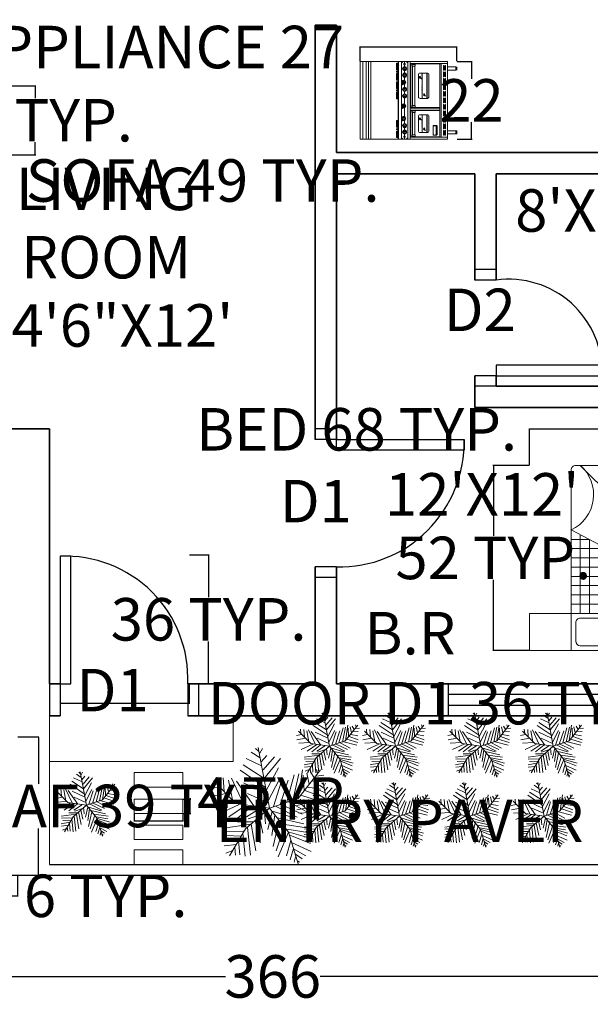
# Model space of a CAD drawing. Units: inches. Extents: x 774 to 1314, y 374 to 930.
# Tile 2 of 5: x 976 to 1137, y 374 to 652. Entities that reach past the tile are written whole.
import ezdxf
from ezdxf.enums import TextEntityAlignment as Align

# ---------------------------------------------------------------- set-up
doc = ezdxf.new("R2010")
doc.units = ezdxf.units.IN
doc.header["$MEASUREMENT"] = 0
for name, color, linetype, lineweight in [('A-ANNO-DIMS', 2, 'Continuous', 18), ('A-ANNO-TEXT', 2, 'Continuous', 18), ('A-AREA-IDEN', 2, 'Continuous', 18), ('A-DOOR', 6, 'Continuous', 25), ('A-EQPM', 9, 'Continuous', 18), ('A-FURN', 8, 'Continuous', 18), ('A-GLAZ', 4, 'Continuous', 18), ('A-WALL', 1, 'Continuous', 35), ('C-PROP', 3, 'Continuous', 25), ('L-PAVE', 32, 'Continuous', 18), ('L-PLNT', 3, 'Continuous', 13)]:
    doc.layers.add(name, color=color, linetype=linetype, lineweight=lineweight)
doc.layers.add('Layer4', color=4, linetype='Continuous')
doc.styles.get("Standard").update_dxf_attribs({"font": 'arial.ttf'})
doc.dimstyles.get("Standard").update_dxf_attribs({"dimtxt": 12, "dimasz": 0.18, "dimexe": 0.18, "dimexo": 0.0625, "dimgap": 0.09, "dimtad": 0, "dimtih": 1, "dimtoh": 1, "dimdec": 0, "dimzin": 0, "dimdsep": 46, "dimlunit": 4, "dimtxsty": 'Standard', "dimcen": 0.09, "dimadec": 0, "dimazin": 0, "dimtfac": 1, "dimtdec": 0, "dimtofl": 0, "dimtmove": 0, "dimatfit": 3, "dimfxl": 1, "dimtolj": 1, "dimtzin": 0, "dimarcsym": 0})

# ---------------------------------------------------------------- blocks, each defined once
blk = doc.blocks.new('tr')
at = {"layer": 'Layer4'}
for p, q in [((9, 66), (0, 66)), ((9, 63), (0, 63)), ((0, 63), (0, 3)), ((3, 63), (3, 3)), ((6, 3), (6, 63)), ((9, 3), (9, 63)), ((0, 3), (9, 3)), ((0, 0), (9, 0))]:
    blk.add_line(p, q, dxfattribs=at)
blk = doc.blocks.new('A$C4CBC1980')
for p, q in [((0.45, 2), (0, 2)), ((0, 2), (0, 1.6)), ((0, 2), (2.6, 2)), ((2.15, 2), (0.45, 2)), ((0.45, 2), (0.45, 0.05)), ((0.45, 0.05), (0.45, 2)), ((1.225, 1.95), (0.55, 1.95)), ((2.05, 1.95), (1.375, 1.95)), ((2.6, 2), (2.025, 2)), ((2.15, 0.05), (2.15, 2)), ((2.6, 1.6), (2.6, 2)), ((0.5, 1.9), (0.5, 1.7)), ((1.275, 1.7), (1.275, 1.9)), ((1.325, 1.7), (1.325, 1.9)), ((2.1, 1.7), (2.1, 1.9)), ((2.6, 1.6), (0, 1.6)), ((0.45, 1.6), (2.05, 0)), ((0.451, 1.6), (2.15, 0.697)), ((1.225, 1.65), (0.55, 1.65)), ((2.15, 1.6), (0.587, 1.6)), ((0.65, 1.494), (0.65, 1.6)), ((0.75, 1.441), (0.75, 1.6)), ((0.85, 1.388), (0.85, 1.6)), ((0.95, 1.335), (0.95, 1.6)), ((1.05, 1.282), (1.05, 1.6)), ((1.15, 1.229), (1.15, 1.6)), ((1.25, 1.176), (1.25, 1.6)), ((1.35, 1.122), (1.35, 1.6)), ((2.05, 1.65), (1.375, 1.65)), ((1.45, 1.069), (1.45, 1.6)), ((1.55, 1.016), (1.55, 1.6)), ((1.65, 0.986), (1.65, 1.6)), ((1.75, 0.91), (1.75, 1.6)), ((1.85, 0.857), (1.85, 1.6)), ((1.95, 0.804), (1.95, 1.6)), ((2.05, 0.751), (2.05, 1.6)), ((2.15, 1.5), (0.639, 1.5)), ((2.15, 1.4), (0.827, 1.4)), ((2.15, 1.3), (1.016, 1.3)), ((2.15, 1.2), (1.204, 1.2)), ((2.15, 1.1), (1.392, 1.1)), ((2.15, 1), (1.58, 1)), ((2.15, 0.9), (1.769, 0.9)), ((2.15, 0.8), (1.957, 0.8)), ((0.5, 0), (2.1, 0))]:
    blk.add_line(p, q)
for centre, radius, start, end in [((0.55, 1.9), 0.05, 90, 180), ((1.225, 1.9), 0.05, 0, 90), ((1.375, 1.9), 0.05, 90, 180), ((2.05, 1.9), 0.05, 0, 90), ((0.55, 1.7), 0.05, 180, 270), ((1.225, 1.7), 0.05, 270, 0), ((1.375, 1.7), 0.05, 180, 270), ((2.05, 1.7), 0.05, 270, 0), ((2.327, 0.316), 0.421, 114.9633, 228.7161), ((0.5, 0.05), 0.05, 180, 270), ((0.5, 0.05), 0.05, 180, 270), ((2.1, 0.05), 0.05, 270, 0)]:
    blk.add_arc(centre, radius, start, end)
blk = doc.blocks.new('33')
at = {"color": 0}
for p, q in [((4799.7, 13825.9), (4704, 13825.9)), ((4704, 13825.9), (4704, 13822.9)), ((4799.7, 13822.9), (4799.7, 13825.9)), ((4799.7, 13818.9), (4704, 13818.9)), ((4799.7, 13815.9), (4704, 13815.9)), ((4799.7, 13812.9), (4704, 13812.9)), ((4706, 13781.2), (4714, 13781.2)), ((4711, 13780.6), (4707, 13780)), ((4707, 13779.7), (4711, 13779.7)), ((4714, 13780.7), (4712, 13780)), ((4712, 13779.7), (4716, 13779.7)), ((4714, 13781.2), (4714, 13780.7)), ((4717, 13779.7), (4721, 13779.7)), ((4718.9, 13781.2), (4727, 13781.2)), ((4718.9, 13781.2), (4718.9, 13780.7)), ((4718.9, 13780.7), (4721, 13780)), ((4722, 13780.6), (4726, 13780)), ((4722, 13779.7), (4726, 13779.7)), ((4753.7, 13781.2), (4761.8, 13781.2)), ((4758.7, 13780.6), (4754.7, 13780)), ((4754.7, 13779.7), (4758.7, 13779.7)), ((4761.8, 13780.7), (4759.7, 13780)), ((4759.7, 13779.7), (4763.7, 13779.7)), ((4761.8, 13781.2), (4761.8, 13780.7)), ((4764.7, 13779.7), (4768.7, 13779.7)), ((4766.6, 13781.2), (4774.7, 13781.2)), ((4766.6, 13781.2), (4766.6, 13780.7)), ((4766.6, 13780.7), (4768.7, 13780)), ((4769.7, 13780.6), (4773.7, 13780)), ((4769.7, 13779.7), (4773.7, 13779.7)), ((4776.7, 13781.2), (4784.8, 13781.2)), ((4781.7, 13780.6), (4777.7, 13780)), ((4777.7, 13779.7), (4781.7, 13779.7)), ((4784.8, 13780.7), (4782.7, 13780)), ((4782.7, 13779.7), (4786.7, 13779.7)), ((4784.8, 13781.2), (4784.8, 13780.7)), ((4787.7, 13779.7), (4791.7, 13779.7)), ((4789.7, 13781.2), (4797.7, 13781.2)), ((4789.7, 13781.2), (4789.7, 13780.7)), ((4789.7, 13780.7), (4791.7, 13780)), ((4792.7, 13780.6), (4796.7, 13780)), ((4792.7, 13779.7), (4796.7, 13779.7)), ((4706.5, 13771.4), (4704, 13771.4)), ((4704, 13767.4), (4799.7, 13767.4)), ((4704, 13764.4), (4799.7, 13764.4)), ((4710.4, 13771.4), (4708, 13771.4)), ((4712.9, 13773.9), (4712.9, 13774.4)), ((4718.4, 13771.4), (4715.4, 13771.4)), ((4720.9, 13773.9), (4720.9, 13774.4)), ((4727.3, 13771.4), (4723.4, 13771.4)), ((4729.6, 13774.9), (4729.6, 13775.4)), ((4742.7, 13771.4), (4731.9, 13771.4)), ((4745, 13774.9), (4745, 13775.4)), ((4754.9, 13771.4), (4747.3, 13771.4)), ((4757.4, 13773.9), (4757.4, 13774.4)), ((4762.9, 13771.4), (4759.9, 13771.4)), ((4765.4, 13773.9), (4765.4, 13774.4)), ((4771.8, 13771.4), (4767.9, 13771.4)), ((4774.1, 13774.9), (4774.1, 13775.4)), ((4780.4, 13771.4), (4776.4, 13771.4)), ((4782.9, 13773.9), (4782.9, 13774.4)), ((4788.4, 13771.4), (4785.4, 13771.4)), ((4790.9, 13773.9), (4790.9, 13774.4)), ((4795.7, 13771.4), (4793.4, 13771.4)), ((4799.7, 13771.4), (4797.2, 13771.4)), ((4730.3, 13753.5), (4727.4, 13750.7)), ((4729.1, 13753.5), (4727.9, 13752.2)), ((4730.4, 13752.5), (4729.7, 13751.7)), ((4781.4, 13753.5), (4778.5, 13750.7)), ((4780.3, 13753.5), (4779, 13752.2)), ((4781.6, 13752.5), (4780.8, 13751.7)), ((4712.2, 13749.9), (4734.2, 13749.9)), ((4712.2, 13749.7), (4734.2, 13749.7)), ((4712.2, 13743.9), (4734.2, 13743.9)), ((4712.2, 13743.7), (4734.2, 13743.7)), ((4717.7, 13748.3), (4714.9, 13745.5)), ((4716.6, 13748.2), (4715.3, 13747)), ((4717.9, 13747.3), (4717.1, 13746.5)), ((4754.4, 13749.9), (4785.4, 13749.9)), ((4754.4, 13749.7), (4785.4, 13749.7)), ((4754.4, 13743.9), (4785.4, 13743.9)), ((4754.4, 13743.7), (4785.4, 13743.7)), ((4759.8, 13748.3), (4757, 13745.5)), ((4758.7, 13748.2), (4757.4, 13747)), ((4760, 13747.3), (4759.2, 13746.5))]:
    blk.add_line(p, q, dxfattribs=at)
for points in [[(4799.7, 13778.9), (4799.7, 13822.9), (4704, 13822.9), (4704, 13778.9)], [(4798.7, 13778.9), (4798.7, 13779.2), (4705, 13779.2), (4705, 13778.9)], [(4706, 13779.2), (4706, 13781.2), (4707, 13781.2), (4707, 13779.2)], [(4711, 13779.2), (4711, 13781.2), (4712, 13781.2), (4712, 13779.2)], [(4716, 13779.2), (4716, 13781.2), (4717, 13781.2), (4717, 13779.2)], [(4721, 13779.2), (4721, 13781.2), (4722, 13781.2), (4722, 13779.2)], [(4726, 13779.2), (4726, 13781.2), (4727, 13781.2), (4727, 13779.2)], [(4753.7, 13779.2), (4753.7, 13781.2), (4754.7, 13781.2), (4754.7, 13779.2)], [(4758.7, 13779.2), (4758.7, 13781.2), (4759.7, 13781.2), (4759.7, 13779.2)], [(4763.7, 13779.2), (4763.7, 13781.2), (4764.7, 13781.2), (4764.7, 13779.2)], [(4768.7, 13779.2), (4768.7, 13781.2), (4769.7, 13781.2), (4769.7, 13779.2)], [(4773.7, 13779.2), (4773.7, 13781.2), (4774.7, 13781.2), (4774.7, 13779.2)], [(4776.7, 13779.2), (4776.7, 13781.2), (4777.7, 13781.2), (4777.7, 13779.2)], [(4781.7, 13779.2), (4781.7, 13781.2), (4782.7, 13781.2), (4782.7, 13779.2)], [(4786.7, 13779.2), (4786.7, 13781.2), (4787.7, 13781.2), (4787.7, 13779.2)], [(4791.7, 13779.2), (4791.7, 13781.2), (4792.7, 13781.2), (4792.7, 13779.2)], [(4796.7, 13779.2), (4796.7, 13781.2), (4797.7, 13781.2), (4797.7, 13779.2)]]:
    blk.add_lwpolyline(points, dxfattribs=at)
for points in [[(4799.7, 13778.9), (4704, 13778.9), (4704, 13775.4), (4799.7, 13775.4)], [(4799.7, 13775.4), (4704, 13775.4), (4704, 13767.4), (4799.7, 13767.4)], [(4704, 13767.4), (4799.7, 13767.4), (4799.7, 13764.4), (4704, 13764.4)], [(4706.5, 13764.4), (4704, 13764.4), (4704, 13718.4), (4706.5, 13718.4)], [(4705, 13774.5), (4705.1, 13774.5), (4705.2, 13774.5), (4705.1, 13774.4), (4705.1, 13774.3), (4705.1, 13774.2), (4705, 13774.3), (4704.8, 13774.3), (4704.8, 13774.4), (4704.9, 13774.4), (4704.9, 13774.6), (4704.9, 13774.6)], [(4705.1, 13768.4), (4705.1, 13768.6), (4705.1, 13768.6), (4705, 13768.5), (4704.8, 13768.5), (4704.8, 13768.5), (4704.9, 13768.4), (4704.9, 13768.3), (4704.9, 13768.2), (4705, 13768.3), (4705.1, 13768.3), (4705.2, 13768.4)], [(4708, 13772.2), (4706.5, 13772.2), (4706.5, 13770.7), (4708, 13770.7)], [(4740, 13764.4), (4742.5, 13764.4), (4742.5, 13727.9), (4740, 13727.9)], [(4795.7, 13772.2), (4797.2, 13772.2), (4797.2, 13770.7), (4795.7, 13770.7)], [(4799.7, 13718.4), (4797.2, 13718.4), (4797.2, 13764.4), (4799.7, 13764.4)], [(4798.7, 13774.4), (4798.6, 13774.4), (4798.6, 13774.3), (4798.7, 13774.3), (4798.8, 13774.2), (4798.9, 13774.3), (4798.8, 13774.4), (4798.9, 13774.5), (4798.9, 13774.5), (4798.8, 13774.5), (4798.7, 13774.6), (4798.6, 13774.6)], [(4798.7, 13768.3), (4798.6, 13768.3), (4798.6, 13768.3), (4798.6, 13768.4), (4798.6, 13768.5), (4798.6, 13768.6), (4798.7, 13768.5), (4798.8, 13768.6), (4798.9, 13768.5), (4798.8, 13768.4), (4798.9, 13768.3), (4798.8, 13768.3)], [(4707, 13763.7), (4739.5, 13763.7), (4739.5, 13727.9), (4707, 13727.9)], [(4707.5, 13758.2), (4709.5, 13758.2), (4709.5, 13762.2), (4707.5, 13762.2)], [(4737, 13758.7), (4709.5, 13758.7), (4709.5, 13761.7), (4737, 13761.7)], [(4739, 13758.2), (4737, 13758.2), (4737, 13762.2), (4739, 13762.2)], [(4796.7, 13763.7), (4743, 13763.7), (4743, 13727.9), (4796.7, 13727.9)], [(4743.5, 13758.2), (4745.5, 13758.2), (4745.5, 13762.2), (4743.5, 13762.2)], [(4794.2, 13758.7), (4745.5, 13758.7), (4745.5, 13761.7), (4794.2, 13761.7)], [(4796.2, 13758.2), (4794.2, 13758.2), (4794.2, 13762.2), (4796.2, 13762.2)], [(4797.2, 13726.4), (4706.5, 13726.4), (4706.5, 13727.9), (4797.2, 13727.9)], [(4706.5, 13726.4), (4797.2, 13726.4), (4797.2, 13718.4), (4706.5, 13718.4)], [(4714.5, 13708.2), (4710.5, 13708.2), (4710.5, 13718.4), (4714.5, 13718.4)], [(4789.2, 13708.2), (4793.2, 13708.2), (4793.2, 13718.4), (4789.2, 13718.4)], [(4714.5, 13707.2), (4710.5, 13707.2), (4710.5, 13706.9), (4714.5, 13706.9)], [(4710.7, 13708.2), (4714.2, 13708.2), (4714.2, 13707.2), (4710.7, 13707.2)], [(4789.2, 13707.2), (4793.2, 13707.2), (4793.2, 13706.9), (4789.2, 13706.9)], [(4793, 13708.2), (4789.5, 13708.2), (4789.5, 13707.2), (4793, 13707.2)]]:
    blk.add_lwpolyline(points, close=True, dxfattribs=at)
for points in [[(4732.2, 13754.4), (4714.2, 13754.4, 0.414214), (4712.2, 13752.4), (4712.2, 13743.4, 0.414214), (4714.2, 13741.4), (4732.2, 13741.4, 0.414214), (4734.2, 13743.4), (4734.2, 13752.4, 0.414214)], [(4783.4, 13754.4), (4756.4, 13754.4, 0.414214), (4754.4, 13752.4), (4754.4, 13743.4, 0.414214), (4756.4, 13741.4), (4783.4, 13741.4, 0.414214), (4785.4, 13743.4), (4785.4, 13752.4, 0.414214)], [(4720, 13731.4), (4710, 13731.4, -0.414214), (4709, 13732.4), (4709, 13735.4, -0.414214), (4710, 13736.4), (4720, 13736.4, -0.414214), (4721, 13735.4), (4721, 13732.4, -0.414214)], [(4710, 13736.2), (4720, 13736.2, -0.414214), (4720.7, 13735.4), (4720.7, 13733.4, -0.414214), (4720, 13732.7), (4710, 13732.7, -0.414214), (4709.2, 13733.4), (4709.2, 13735.4, -0.414214)], [(4714.3, 13723.7), (4709.4, 13723.7, 0.284079), (4709, 13723.4), (4708.9, 13723.2), (4714.9, 13723.2), (4714.8, 13723.4, 0.284079)], [(4714.3, 13721.7), (4709.4, 13721.7, 0.284079), (4709, 13721.4), (4708.9, 13721.2), (4714.9, 13721.2), (4714.8, 13721.4, 0.284079)], [(4722.3, 13723.7), (4717.4, 13723.7, 0.284079), (4717, 13723.4), (4716.9, 13723.2), (4722.9, 13723.2), (4722.8, 13723.4, 0.284079)], [(4722.3, 13721.7), (4717.4, 13721.7, 0.284079), (4717, 13721.4), (4716.9, 13721.2), (4722.9, 13721.2), (4722.8, 13721.4, 0.284079)], [(4730.3, 13723.7), (4725.4, 13723.7, 0.284079), (4725, 13723.4), (4724.9, 13723.2), (4730.9, 13723.2), (4730.8, 13723.4, 0.284079)], [(4730.3, 13721.7), (4725.4, 13721.7, 0.284079), (4725, 13721.4), (4724.9, 13721.2), (4730.9, 13721.2), (4730.8, 13721.4, 0.284079)], [(4738.3, 13723.7), (4733.4, 13723.7, 0.284079), (4733, 13723.4), (4732.9, 13723.2), (4738.9, 13723.2), (4738.8, 13723.4, 0.284079)], [(4738.3, 13721.7), (4733.4, 13721.7, 0.284079), (4733, 13721.4), (4732.9, 13721.2), (4738.9, 13721.2), (4738.8, 13721.4, 0.284079)], [(4746.3, 13723.7), (4741.4, 13723.7, 0.284079), (4741, 13723.4), (4740.9, 13723.2), (4746.9, 13723.2), (4746.8, 13723.4, 0.284079)], [(4746.3, 13721.7), (4741.4, 13721.7, 0.284079), (4741, 13721.4), (4740.9, 13721.2), (4746.9, 13721.2), (4746.8, 13721.4, 0.284079)], [(4754.3, 13723.7), (4749.4, 13723.7, 0.284079), (4749, 13723.4), (4748.9, 13723.2), (4754.9, 13723.2), (4754.8, 13723.4, 0.284079)], [(4754.3, 13721.7), (4749.4, 13721.7, 0.284079), (4749, 13721.4), (4748.9, 13721.2), (4754.9, 13721.2), (4754.8, 13721.4, 0.284079)], [(4762.3, 13723.7), (4757.4, 13723.7, 0.284079), (4757, 13723.4), (4756.9, 13723.2), (4762.9, 13723.2), (4762.8, 13723.4, 0.284079)], [(4762.3, 13721.7), (4757.4, 13721.7, 0.284079), (4757, 13721.4), (4756.9, 13721.2), (4762.9, 13721.2), (4762.8, 13721.4, 0.284079)], [(4770.3, 13723.7), (4765.4, 13723.7, 0.284079), (4765, 13723.4), (4764.9, 13723.2), (4770.9, 13723.2), (4770.8, 13723.4, 0.284079)], [(4770.3, 13721.7), (4765.4, 13721.7, 0.284079), (4765, 13721.4), (4764.9, 13721.2), (4770.9, 13721.2), (4770.8, 13721.4, 0.284079)], [(4778.3, 13723.7), (4773.4, 13723.7, 0.284079), (4773, 13723.4), (4772.9, 13723.2), (4778.9, 13723.2), (4778.8, 13723.4, 0.284079)], [(4778.3, 13721.7), (4773.4, 13721.7, 0.284079), (4773, 13721.4), (4772.9, 13721.2), (4778.9, 13721.2), (4778.8, 13721.4, 0.284079)], [(4786.3, 13723.7), (4781.4, 13723.7, 0.284079), (4781, 13723.4), (4780.9, 13723.2), (4786.9, 13723.2), (4786.8, 13723.4, 0.284079)], [(4786.3, 13721.7), (4781.4, 13721.7, 0.284079), (4781, 13721.4), (4780.9, 13721.2), (4786.9, 13721.2), (4786.8, 13721.4, 0.284079)], [(4794.3, 13723.7), (4789.4, 13723.7, 0.284079), (4789, 13723.4), (4788.9, 13723.2), (4794.9, 13723.2), (4794.8, 13723.4, 0.284079)], [(4794.3, 13721.7), (4789.4, 13721.7, 0.284079), (4789, 13721.4), (4788.9, 13721.2), (4794.9, 13721.2), (4794.8, 13721.4, 0.284079)]]:
    blk.add_lwpolyline(points, format="xyb", close=True, dxfattribs=at)
for centre, radius in [((4705, 13774.4), 0.25), ((4705, 13768.4), 0.25), ((4712.9, 13771.4), 2.5), ((4712.9, 13771.4), 2), ((4720.9, 13771.4), 2.5), ((4720.9, 13771.4), 2), ((4726.8, 13774.2), 0.25), ((4729.6, 13772.4), 2.5), ((4729.6, 13772.4), 2), ((4742.2, 13774.2), 0.25), ((4745, 13772.4), 2.5), ((4745, 13772.4), 2), ((4757.4, 13771.4), 2.5), ((4757.4, 13771.4), 2), ((4765.4, 13771.4), 2.5), ((4765.4, 13771.4), 2), ((4771.3, 13774.2), 0.25), ((4774.1, 13772.4), 2.5), ((4774.1, 13772.4), 2), ((4782.9, 13771.4), 2.5), ((4782.9, 13771.4), 2), ((4790.9, 13771.4), 2.5), ((4790.9, 13771.4), 2), ((4798.7, 13774.4), 0.25), ((4798.7, 13768.4), 0.25)]:
    blk.add_circle(centre, radius, dxfattribs=at)
for centre, radius, start, end in [((4698.4, 13771.4), 13.8, 352.2859, 7.7141), ((4727.3, 13771.4), 13.8, 172.2859, 187.7141), ((4706.4, 13771.4), 13.8, 352.2859, 7.7141), ((4735.3, 13771.4), 13.8, 172.2859, 187.7141), ((4715.2, 13772.4), 13.8, 352.2859, 7.7141), ((4744.1, 13772.4), 13.8, 172.2859, 187.7141), ((4730.6, 13772.4), 13.8, 352.2859, 7.7141), ((4759.4, 13772.4), 13.8, 172.2859, 187.7141), ((4742.9, 13771.4), 13.8, 352.2859, 7.7141), ((4771.8, 13771.4), 13.8, 172.2859, 187.7141), ((4750.9, 13771.4), 13.8, 352.2859, 7.7141), ((4779.8, 13771.4), 13.8, 172.2859, 187.7141), ((4759.7, 13772.4), 13.8, 352.2859, 7.7141), ((4788.6, 13772.4), 13.8, 172.2859, 187.7141), ((4768.4, 13771.4), 13.8, 352.2859, 7.7141), ((4797.3, 13771.4), 13.8, 172.2859, 187.7141), ((4776.4, 13771.4), 13.8, 352.2859, 7.7141), ((4805.3, 13771.4), 13.8, 172.2859, 187.7141), ((4713.2, 13749.9), 0.125, 0, 180), ((4713.2, 13743.9), 0.125, 0, 180), ((4715.2, 13749.9), 0.125, 0, 180), ((4715.2, 13743.9), 0.125, 0, 180), ((4717.2, 13749.9), 0.125, 0, 180), ((4717.2, 13743.9), 0.125, 0, 180), ((4719.2, 13749.9), 0.125, 0, 180), ((4719.2, 13743.9), 0.125, 0, 180), ((4721.2, 13749.9), 0.125, 0, 180), ((4721.2, 13743.9), 0.125, 0, 180), ((4723.2, 13749.9), 0.125, 0, 180), ((4723.2, 13743.9), 0.125, 0, 180), ((4725.2, 13749.9), 0.125, 0, 180), ((4725.2, 13743.9), 0.125, 0, 180), ((4727.2, 13749.9), 0.125, 0, 180), ((4727.2, 13743.9), 0.125, 0, 180), ((4729.2, 13749.9), 0.125, 0, 180), ((4729.2, 13743.9), 0.125, 0, 180), ((4731.2, 13749.9), 0.125, 0, 180), ((4731.2, 13743.9), 0.125, 0, 180), ((4733.2, 13749.9), 0.125, 0, 180), ((4733.2, 13743.9), 0.125, 0, 180), ((4755.9, 13749.9), 0.125, 0, 180), ((4755.9, 13743.9), 0.125, 0, 180), ((4757.9, 13749.9), 0.125, 0, 180), ((4757.9, 13743.9), 0.125, 0, 180), ((4759.9, 13749.9), 0.125, 0, 180), ((4759.9, 13743.9), 0.125, 0, 180), ((4761.9, 13749.9), 0.125, 0, 180), ((4761.9, 13743.9), 0.125, 0, 180), ((4763.9, 13749.9), 0.125, 0, 180), ((4763.9, 13743.9), 0.125, 0, 180), ((4765.9, 13749.9), 0.125, 0, 180), ((4765.9, 13743.9), 0.125, 0, 180), ((4767.9, 13749.9), 0.125, 0, 180), ((4767.9, 13743.9), 0.125, 0, 180), ((4769.9, 13749.9), 0.125, 0, 180), ((4769.9, 13743.9), 0.125, 0, 180), ((4771.9, 13749.9), 0.125, 0, 180), ((4771.9, 13743.9), 0.125, 0, 180), ((4773.9, 13749.9), 0.125, 0, 180), ((4773.9, 13743.9), 0.125, 0, 180), ((4775.9, 13749.9), 0.125, 0, 180), ((4775.9, 13743.9), 0.125, 0, 180), ((4777.9, 13749.9), 0.125, 0, 180), ((4777.9, 13743.9), 0.125, 0, 180), ((4779.9, 13749.9), 0.125, 0, 180), ((4779.9, 13743.9), 0.125, 0, 180), ((4781.9, 13749.9), 0.125, 0, 180), ((4781.9, 13743.9), 0.125, 0, 180), ((4783.9, 13749.9), 0.125, 0, 180), ((4783.9, 13743.9), 0.125, 0, 180)]:
    blk.add_arc(centre, radius, start, end, dxfattribs=at)
blk = doc.blocks.new('*U14')
for p, q in [((-10.186, 53.64), (-13.084, 55.962)), ((0, 0), (-10.5, 57)), ((-9.099, 51.782), (-6.563, 55.962)), ((-7.288, 39.707), (-21.778, 46.673)), ((-8.737, 47.138), (-17.069, 52.711)), ((-7.65, 43.423), (-2.578, 49.46)), ((-5.839, 35.992), (4.667, 48.067)), ((-5.114, 27.632), (10.463, 46.673)), ((-5.114, 28.097), (-24.676, 40.636)), ((-2.941, 16.486), (8.652, 37.85)), ((-48.585, 21.131), (-49.309, 29.026)), ((-43.513, 28.561), (-42.427, 15.558)), ((-35.544, 28.097), (-24.314, 3.947)), ((-3.665, 19.273), (-27.574, 35.527)), ((16.259, 5.805), (23.142, 31.348)), ((22.055, 7.198), (27.489, 32.277)), ((27, 9), (48, 36)), ((27.127, 9.056), (31.112, 35.992)), ((31.836, 30.883), (32.561, 16.486)), ((35.096, 32.741), (37.27, 22.524)), ((38.719, 34.134), (41.979, 28.561)), ((43.791, 29.954), (51.036, 30.883)), ((44.153, 36.456), (45.239, 32.741)), ((-47.498, 19.737), (-55.83, 18.344)), ((-31.5, 4.5), (-52.5, 25.5)), ((-38.442, 26.239), (-34.819, 7.663)), ((-14.533, 2.09), (-30.834, 25.31)), ((-24.314, 23.917), (-2.941, 13.7)), ((-1.129, 6.734), (9.014, 26.704)), ((3.942, 1.625), (11.187, 24.381)), ((10.101, 3.483), (17.708, 26.239)), ((36.183, 19.737), (48.137, 17.88)), ((40.53, 25.775), (48.862, 24.846)), ((-40.615, 13.7), (-55.105, 10.913)), ((-20.691, 13.7), (-1.129, 4.876)), ((29.662, 12.307), (48.137, 6.269)), ((33.285, 16.486), (48.862, 10.913)), ((-33.37, 6.269), (-52.207, 5.34)), ((-28.299, 3.483), (-47.86, -5.805)), ((-21.416, 3.018), (-38.079, -8.128)), ((0, 0), (-31.5, 4.5)), ((-15.982, 2.09), (-30.11, -9.521)), ((0, 0), (-22.5, -19.5)), ((-6.563, 1.161), (-21.416, -8.128)), ((0, 0), (27, 9)), ((0, 0), (18, -22.5)), ((6.478, 1.625), (26.04, -8.592)), ((11.187, 3.483), (30.749, -5.805)), ((18.07, 5.805), (35.096, -3.483)), ((24.229, 7.663), (46.688, 1.625)), ((-6.563, -5.805), (-19.967, -9.985)), ((-9.461, -8.592), (-6.201, -23.453)), ((-4.752, -3.483), (-3.665, -14.629)), ((2.493, -3.019), (-1.491, -20.202)), ((1.769, -2.555), (24.229, -9.521)), ((5.029, -6.27), (2.131, -25.775)), ((7.565, -9.056), (32.198, -14.629)), ((-17.431, -15.094), (-42.789, -18.809)), ((-15.257, -12.772), (-30.11, -12.772)), ((-20.691, -18.345), (-17.793, -44.352)), ((-17.069, -15.094), (-12.721, -40.172)), ((-13.446, -11.378), (-8.737, -32.741)), ((9.014, -11.378), (3.58, -35.992)), ((14.085, -16.951), (6.478, -40.172)), ((12.274, -15.094), (36.907, -18.809)), ((-24.314, -21.596), (-42.427, -22.06)), ((-26.849, -26.24), (-40.253, -25.775)), ((-22.5, -19.5), (-37.5, -45)), ((-25.038, -23.918), (-22.865, -45.281)), ((18.07, -22.524), (8.289, -45.745)), ((16.259, -19.738), (36.183, -22.989)), ((18, -22.5), (27, -52.5)), ((18.433, -22.524), (40.53, -29.026)), ((19.157, -25.311), (38.719, -33.206)), ((-28.299, -29.026), (-42.789, -31.348)), ((-30.834, -34.135), (-42.427, -35.528)), ((-32.646, -36.921), (-31.921, -44.352)), ((-29.023, -30.884), (-27.936, -43.887)), ((20.244, -30.419), (15.897, -44.816)), ((21.331, -32.741), (39.081, -40.636)), ((-34.457, -39.708), (-40.978, -42.494)), ((22.78, -37.85), (19.519, -48.532)), ((22.78, -38.314), (34.372, -44.816)), ((24.591, -45.745), (23.142, -50.854)), ((24.591, -43.423), (30.749, -47.603)), ((26.764, -49.925), (28.213, -50.854))]:
    blk.add_line(p, q)
blk = doc.blocks.new('DOOR-SWING-36IN')
blk.add_lwpolyline([(0, 0), (3, 0), (3, 36), (0, 36)], close=True)
blk.add_arc((1.5, 1.5), 34.53, 357.5104, 92.4896)
blk = doc.blocks.new('ENTRY-STEPPING-STONE')
blk.add_lwpolyline([(0, 0), (13.75, 0), (13.75, 4.1), (0, 4.1)], close=True)
blk = doc.blocks.new('*D29')
at = {"layer": 'A-ANNO-DIMS', "color": 0, "lineweight": -2, "transparency": 16777216}
for p, q in [((987.33, 464.5), (987.33, 458.92)), ((1023.76, 464.5), (1023.76, 458.92)), ((987.51, 459.1), (1023.58, 459.1)), ((1023.76, 459.1), (1023.94, 459.1))]:
    blk.add_line(p, q, dxfattribs=at)
at = {"layer": 'A-ANNO-DIMS', "color": 0, "transparency": 16777216}
for points in [[(987.51, 459.13), (987.51, 459.07), (987.33, 459.1)], [(1023.58, 459.13), (1023.58, 459.07), (1023.76, 459.1)]]:
    blk.add_solid(points, dxfattribs=at)
at = {"layer": 'Defpoints', "color": 0, "transparency": 16777216}
for p in [(987.33, 464.57), (1023.76, 464.57), (1023.76, 459.1)]:
    blk.add_point(p, dxfattribs=at)
at = {"layer": 'A-ANNO-DIMS', "color": 0, "transparency": 16777216, "insert": (1093.45, 459.1), "char_height": 12, "attachment_point": 5}
blk.add_mtext('\\A1;DOOR D1 36 TYP.', dxfattribs=at)
blk = doc.blocks.new('*D30')
at = {"layer": 'A-ANNO-DIMS', "color": 0, "lineweight": -2, "transparency": 16777216}
for p, q in [((1023.82, 500.99), (1029.4, 500.99)), ((1029.22, 500.81), (1029.22, 489)), ((1029.22, 464.75), (1029.22, 476.55)), ((1023.82, 464.57), (1029.4, 464.57))]:
    blk.add_line(p, q, dxfattribs=at)
at = {"layer": 'A-ANNO-DIMS', "color": 0, "transparency": 16777216}
for points in [[(1029.19, 500.81), (1029.25, 500.81), (1029.22, 500.99)], [(1029.19, 464.75), (1029.25, 464.75), (1029.22, 464.57)]]:
    blk.add_solid(points, dxfattribs=at)
at = {"layer": 'Defpoints', "color": 0, "transparency": 16777216}
for p in [(1023.76, 500.99), (1029.22, 500.99), (1023.76, 464.57)]:
    blk.add_point(p, dxfattribs=at)
at = {"layer": 'A-ANNO-DIMS', "color": 0, "transparency": 16777216, "insert": (1029.22, 482.78), "char_height": 12, "attachment_point": 5}
blk.add_mtext('\\A1;36 TYP.', dxfattribs=at)
blk = doc.blocks.new('*D33')
at = {"layer": 'A-ANNO-DIMS', "color": 0, "lineweight": -2, "transparency": 16777216}
for p, q in [((975.4, 449.57), (981.36, 449.57)), ((981.18, 449.39), (981.18, 436.36)), ((981.18, 410.75), (981.18, 423.77)), ((975.4, 410.57), (981.36, 410.57))]:
    blk.add_line(p, q, dxfattribs=at)
at = {"layer": 'A-ANNO-DIMS', "color": 0, "transparency": 16777216}
for points in [[(981.15, 449.39), (981.21, 449.39), (981.18, 449.57)], [(981.15, 410.75), (981.21, 410.75), (981.18, 410.57)]]:
    blk.add_solid(points, dxfattribs=at)
at = {"layer": 'Defpoints', "color": 0, "transparency": 16777216}
for p in [(975.33, 449.57), (981.18, 449.57), (975.33, 410.57)]:
    blk.add_point(p, dxfattribs=at)
at = {"layer": 'A-ANNO-DIMS', "color": 0, "transparency": 16777216, "insert": (981.18, 430.07), "char_height": 12, "attachment_point": 5}
blk.add_mtext('\\A1;GATE LEAF 39 TYP.', dxfattribs=at)
blk = doc.blocks.new('*D34')
at = {"layer": 'A-ANNO-DIMS', "color": 0, "lineweight": -2, "transparency": 16777216}
for p, q in [((969.33, 410.5), (969.33, 404.54)), ((975.33, 410.5), (975.33, 404.54)), ((969.51, 404.72), (975.15, 404.72)), ((975.33, 404.72), (975.51, 404.72))]:
    blk.add_line(p, q, dxfattribs=at)
at = {"layer": 'A-ANNO-DIMS', "color": 0, "transparency": 16777216}
for points in [[(969.51, 404.75), (969.51, 404.69), (969.33, 404.72)], [(975.15, 404.75), (975.15, 404.69), (975.33, 404.72)]]:
    blk.add_solid(points, dxfattribs=at)
at = {"layer": 'Defpoints', "color": 0, "transparency": 16777216}
for p in [(969.33, 410.57), (975.33, 410.57), (975.33, 404.72)]:
    blk.add_point(p, dxfattribs=at)
at = {"layer": 'A-ANNO-DIMS', "color": 0, "transparency": 16777216, "insert": (1000.18, 404.72), "char_height": 12, "attachment_point": 5}
blk.add_mtext('\\A1;6 TYP.', dxfattribs=at)
blk = doc.blocks.new('*D35')
at = {"layer": 'A-ANNO-DIMS', "color": 0, "lineweight": -2, "transparency": 16777216}
for p, q in [((1008.19, 427.87), (1008.19, 425.69)), ((1008.37, 425.87), (1021.76, 425.87)), ((1021.94, 427.87), (1021.94, 425.69)), ((1021.94, 425.87), (1022.12, 425.87))]:
    blk.add_line(p, q, dxfattribs=at)
at = {"layer": 'A-ANNO-DIMS', "color": 0, "transparency": 16777216}
for points in [[(1008.37, 425.9), (1008.37, 425.84), (1008.19, 425.87)], [(1021.76, 425.9), (1021.76, 425.84), (1021.94, 425.87)]]:
    blk.add_solid(points, dxfattribs=at)
at = {"layer": 'Defpoints', "color": 0, "transparency": 16777216}
for p in [(1008.19, 427.93), (1021.94, 427.93), (1021.94, 425.87)]:
    blk.add_point(p, dxfattribs=at)
at = {"layer": 'A-ANNO-DIMS', "color": 0, "transparency": 16777216, "insert": (1112.58, 425.87), "char_height": 12, "attachment_point": 5}
blk.add_mtext('\\A1;ENTRY PAVER 14 TYP.', dxfattribs=at)
blk = doc.blocks.new('*D36')
at = {"layer": 'A-ANNO-DIMS', "color": 0, "lineweight": -2, "transparency": 16777216}
for p, q in [((1022, 432.03), (1024.18, 432.03)), ((1024, 432.03), (1024, 432.21)), ((1024, 432.21), (1024.18, 432.21)), ((1024, 428.11), (1024, 431.85)), ((1022, 427.93), (1024.18, 427.93))]:
    blk.add_line(p, q, dxfattribs=at)
at = {"layer": 'A-ANNO-DIMS', "color": 0, "transparency": 16777216}
for points in [[(1023.97, 431.85), (1024.03, 431.85), (1024, 432.03)], [(1023.97, 428.11), (1024.03, 428.11), (1024, 427.93)]]:
    blk.add_solid(points, dxfattribs=at)
at = {"layer": 'Defpoints', "color": 0, "transparency": 16777216}
for p in [(1021.94, 432.03), (1024, 432.03), (1021.94, 427.93)]:
    blk.add_point(p, dxfattribs=at)
at = {"layer": 'A-ANNO-DIMS', "color": 0, "transparency": 16777216, "insert": (1049.06, 432.21), "char_height": 12, "attachment_point": 5}
blk.add_mtext('\\A1;4 TYP.', dxfattribs=at)
blk = doc.blocks.new('*D37')
at = {"layer": 'A-ANNO-DIMS', "color": 0, "lineweight": -2, "transparency": 16777216}
for p, q in [((924.33, 613.89), (924.33, 606.48)), ((972.96, 613.89), (972.96, 606.48)), ((924.51, 606.66), (972.78, 606.66)), ((972.96, 606.66), (973.14, 606.66))]:
    blk.add_line(p, q, dxfattribs=at)
at = {"layer": 'A-ANNO-DIMS', "color": 0, "transparency": 16777216}
for points in [[(924.51, 606.69), (924.51, 606.63), (924.33, 606.66)], [(972.78, 606.69), (972.78, 606.63), (972.96, 606.66)]]:
    blk.add_solid(points, dxfattribs=at)
at = {"layer": 'Defpoints', "color": 0, "transparency": 16777216}
for p in [(924.33, 613.95), (972.96, 613.95), (972.96, 606.66)]:
    blk.add_point(p, dxfattribs=at)
at = {"layer": 'A-ANNO-DIMS', "color": 0, "transparency": 16777216, "insert": (1027.55, 606.66), "char_height": 12, "attachment_point": 5}
blk.add_mtext('\\A1;SOFA 49 TYP.', dxfattribs=at)
blk = doc.blocks.new('*D38')
at = {"layer": 'A-ANNO-DIMS', "color": 0, "lineweight": -2, "transparency": 16777216}
for p, q in [((973.02, 633.4), (980.43, 633.4)), ((980.25, 633.22), (980.25, 629.89)), ((980.25, 614.13), (980.25, 617.46)), ((973.02, 613.95), (980.43, 613.95))]:
    blk.add_line(p, q, dxfattribs=at)
at = {"layer": 'A-ANNO-DIMS', "color": 0, "transparency": 16777216}
for points in [[(980.22, 633.22), (980.28, 633.22), (980.25, 633.4)], [(980.22, 614.13), (980.28, 614.13), (980.25, 613.95)]]:
    blk.add_solid(points, dxfattribs=at)
at = {"layer": 'Defpoints', "color": 0, "transparency": 16777216}
for p in [(972.96, 633.4), (980.25, 633.4), (972.96, 613.95)]:
    blk.add_point(p, dxfattribs=at)
at = {"layer": 'A-ANNO-DIMS', "color": 0, "transparency": 16777216, "insert": (980.25, 623.68), "char_height": 12, "attachment_point": 5}
blk.add_mtext('\\A1;19 TYP.', dxfattribs=at)
blk = doc.blocks.new('*D39')
at = {"layer": 'A-ANNO-DIMS', "color": 0, "lineweight": -2, "transparency": 16777216}
for p, q in [((1119.75, 526.29), (1119.75, 536.6)), ((1187.64, 526.29), (1187.64, 536.6)), ((1119.75, 536.42), (1119.57, 536.42)), ((1187.46, 536.42), (1119.93, 536.42))]:
    blk.add_line(p, q, dxfattribs=at)
at = {"layer": 'A-ANNO-DIMS', "color": 0, "transparency": 16777216}
for points in [[(1119.93, 536.45), (1119.93, 536.39), (1119.75, 536.42)], [(1187.46, 536.45), (1187.46, 536.39), (1187.64, 536.42)]]:
    blk.add_solid(points, dxfattribs=at)
at = {"layer": 'Defpoints', "color": 0, "transparency": 16777216}
for p in [(1119.75, 536.42), (1119.75, 526.23), (1187.64, 526.23)]:
    blk.add_point(p, dxfattribs=at)
at = {"layer": 'A-ANNO-DIMS', "color": 0, "transparency": 16777216, "insert": (1070.98, 536.42), "char_height": 12, "attachment_point": 5}
blk.add_mtext('\\A1;BED 68 TYP.', dxfattribs=at)
blk = doc.blocks.new('*D40')
at = {"layer": 'A-ANNO-DIMS', "color": 0, "lineweight": -2, "transparency": 16777216}
for p, q in [((1119.69, 526.23), (1109.39, 526.23)), ((1109.57, 526.05), (1109.57, 506.34)), ((1109.57, 474.19), (1109.57, 493.9)), ((1119.69, 474.01), (1109.39, 474.01))]:
    blk.add_line(p, q, dxfattribs=at)
at = {"layer": 'A-ANNO-DIMS', "color": 0, "transparency": 16777216}
for points in [[(1109.54, 526.05), (1109.6, 526.05), (1109.57, 526.23)], [(1109.54, 474.19), (1109.6, 474.19), (1109.57, 474.01)]]:
    blk.add_solid(points, dxfattribs=at)
at = {"layer": 'Defpoints', "color": 0, "transparency": 16777216}
for p in [(1119.75, 526.23), (1109.57, 474.01), (1119.75, 474.01)]:
    blk.add_point(p, dxfattribs=at)
at = {"layer": 'A-ANNO-DIMS', "color": 0, "transparency": 16777216, "insert": (1109.57, 500.12), "char_height": 12, "attachment_point": 5}
blk.add_mtext('\\A1;52 TYP.', dxfattribs=at)
blk = doc.blocks.new('*D51')
at = {"layer": 'A-ANNO-DIMS', "color": 0, "lineweight": -2, "transparency": 16777216}
for p, q in [((1072.03, 644.35), (1071.85, 644.35)), ((1072.03, 640.32), (1072.03, 644.53)), ((1099.12, 644.35), (1072.21, 644.35)), ((1099.3, 640.32), (1099.3, 644.53))]:
    blk.add_line(p, q, dxfattribs=at)
at = {"layer": 'A-ANNO-DIMS', "color": 0, "transparency": 16777216}
for points in [[(1072.21, 644.38), (1072.21, 644.32), (1072.03, 644.35)], [(1099.12, 644.38), (1099.12, 644.32), (1099.3, 644.35)]]:
    blk.add_solid(points, dxfattribs=at)
at = {"layer": 'Defpoints', "color": 0, "transparency": 16777216}
for p in [(1072.03, 644.35), (1072.03, 640.25), (1099.3, 640.25)]:
    blk.add_point(p, dxfattribs=at)
at = {"layer": 'A-ANNO-DIMS', "color": 0, "transparency": 16777216, "insert": (1013.43, 644.35), "char_height": 12, "attachment_point": 5}
blk.add_mtext('\\A1;APPLIANCE 27', dxfattribs=at)
blk = doc.blocks.new('*D52')
at = {"layer": 'A-ANNO-DIMS', "color": 0, "lineweight": -2, "transparency": 16777216}
for p, q in [((1099.37, 640.25), (1103.58, 640.25)), ((1103.4, 640.07), (1103.4, 635.39)), ((1103.4, 618.49), (1103.4, 623.17)), ((1099.37, 618.31), (1103.58, 618.31))]:
    blk.add_line(p, q, dxfattribs=at)
at = {"layer": 'A-ANNO-DIMS', "color": 0, "transparency": 16777216}
for points in [[(1103.37, 640.07), (1103.43, 640.07), (1103.4, 640.25)], [(1103.37, 618.49), (1103.43, 618.49), (1103.4, 618.31)]]:
    blk.add_solid(points, dxfattribs=at)
at = {"layer": 'Defpoints', "color": 0, "transparency": 16777216}
for p in [(1099.3, 640.25), (1103.4, 640.25), (1099.3, 618.31)]:
    blk.add_point(p, dxfattribs=at)
at = {"layer": 'A-ANNO-DIMS', "color": 0, "transparency": 16777216, "insert": (1103.4, 629.28), "char_height": 12, "attachment_point": 5}
blk.add_mtext('\\A1;22', dxfattribs=at)
blk = doc.blocks.new('*D53')
at = {"layer": 'A-ANNO-DIMS', "color": 0, "lineweight": -2, "transparency": 16777216}
for p, q in [((864.33, 410.5), (864.33, 381.78)), ((1230.33, 410.5), (1230.33, 381.78)), ((864.51, 381.96), (1034, 381.96)), ((1230.15, 381.96), (1060.67, 381.96))]:
    blk.add_line(p, q, dxfattribs=at)
at = {"layer": 'A-ANNO-DIMS', "color": 0, "transparency": 16777216}
for points in [[(864.51, 381.99), (864.51, 381.93), (864.33, 381.96)], [(1230.15, 381.99), (1230.15, 381.93), (1230.33, 381.96)]]:
    blk.add_solid(points, dxfattribs=at)
at = {"layer": 'Defpoints', "color": 0, "transparency": 16777216}
for p in [(864.33, 410.57), (1230.33, 410.57), (1230.33, 381.96)]:
    blk.add_point(p, dxfattribs=at)
at = {"layer": 'A-ANNO-DIMS', "color": 0, "transparency": 16777216, "insert": (1047.33, 381.96), "char_height": 12, "attachment_point": 5}
blk.add_mtext('\\A1;366', dxfattribs=at)

msp = doc.modelspace()

# ---------------------------------------------------------------- linework, layer by layer
at = {"layer": 'A-DOOR'}
for p, q in [((1110.3347, 581.5656), (1104.3347, 581.5656)), ((1110.3347, 578.5656), (1104.3347, 578.5656)), ((1110.3347, 551.5656), (1104.3347, 551.5656)), ((1110.3347, 548.5656), (1104.3347, 548.5656)), ((1065.3347, 536.5656), (1059.3347, 536.5656)), ((1065.3347, 533.5656), (1059.3347, 533.5656)), ((1065.3347, 497.5656), (1059.3347, 497.5656)), ((1065.3347, 494.5656), (1059.3347, 494.5656)), ((984.3347, 464.5656), (984.3347, 455.5656)), ((987.3347, 464.5656), (987.3347, 455.5656)), ((1023.3347, 464.5656), (1023.3347, 455.5656)), ((1026.3347, 464.5656), (1026.3347, 455.5656))]:
    msp.add_line(p, q, dxfattribs=at)
for points in [[(1110.3347, 551.5656), (1140.3347, 551.5656), (1140.3347, 554.5656), (1110.3347, 554.5656)], [(1065.3347, 533.5656), (1101.3347, 533.5656), (1101.3347, 530.5656), (1065.3347, 530.5656)]]:
    msp.add_lwpolyline(points, close=True, dxfattribs=at)
for centre, radius, start, end in [((1113.8597, 552.3156), 26.4856, 358.377324, 97.648251), ((1066.0847, 532.8156), 35.258, 268.781125, 1.218875)]:
    msp.add_arc(centre, radius, start, end, dxfattribs=at)
at = {"layer": 'A-WALL'}
for p, q in [((1065.3347, 650.5656), (1059.3347, 650.5656)), ((1065.3347, 650.5656), (1059.3347, 650.5656)), ((1167.3347, 614.5656), (1065.3347, 614.5656)), ((1068.3347, 614.5656), (1065.3347, 614.5656)), ((1104.3347, 608.5656), (1065.3347, 608.5656)), ((1104.3347, 608.5656), (1098.3347, 608.5656)), ((1104.3347, 578.5656), (1104.3347, 608.5656)), ((1206.3347, 608.5656), (1110.3347, 608.5656)), ((1110.3347, 578.5656), (1110.3347, 608.5656)), ((1104.3347, 542.5656), (1104.3347, 551.5656)), ((1110.3347, 548.5656), (1110.3347, 551.5656)), ((1206.3347, 548.5656), (1110.3347, 548.5656)), ((1206.3347, 542.5656), (1104.3347, 542.5656)), ((984.3347, 536.5656), (900.3347, 536.5656)), ((984.3347, 464.5656), (984.3347, 536.5656)), ((987.3347, 464.5656), (984.3347, 464.5656)), ((987.3347, 464.5656), (984.3347, 464.5656)), ((1044.3347, 464.5656), (1023.3347, 464.5656)), ((1059.3347, 464.5656), (1023.3347, 464.5656)), ((1206.3347, 464.5656), (1065.3347, 464.5656)), ((987.3347, 455.5656), (984.3347, 455.5656)), ((1215.3347, 455.5656), (1023.3347, 455.5656))]:
    msp.add_line(p, q, dxfattribs=at)
for points in [[(1059.3347, 533.5656), (1059.3347, 650.5656)], [(1065.3347, 614.5656), (1065.3347, 650.5656)], [(1065.3347, 533.5656), (1065.3347, 608.5656)], [(1059.3347, 464.5656), (1059.3347, 497.5656)], [(1065.3347, 464.5656), (1065.3347, 497.5656)]]:
    msp.add_lwpolyline(points, dxfattribs=at)
at = {"layer": 'C-PROP'}
msp.add_lwpolyline([(864.3347, 410.5656), (1230.3347, 410.5656), (1230.3347, 896.5656), (864.3347, 896.5656)], close=True, dxfattribs=at)
for points in [[(984.3347, 413.5656), (1194.3347, 413.5656)], [(984.3347, 413.5656), (1044.3347, 413.5656)], [(984.3347, 413.5656), (1044.3347, 413.5656)]]:
    msp.add_lwpolyline(points, dxfattribs=at)
at = {"layer": 'L-PAVE'}
for p, q in [((984.3347, 413.5656), (984.3347, 455.5656)), ((1036.17, 455.5656), (1036.17, 442.6323)), ((1036.17, 442.6323), (984.3347, 442.6323))]:
    msp.add_line(p, q, dxfattribs=at)

# ---------------------------------------------------------------- block references
at = {"layer": 'A-DOOR'}
msp.add_blockref('DOOR-SWING-36IN', (987.335, 464.566), dxfattribs=at)
at = {"layer": 'A-EQPM', "xscale": 0.2292227651302432, "yscale": 0.2292227651302432, "zscale": 0.2292227651302432, "rotation": 90}
msp.add_blockref('33', (4241.2419, -459.9551), dxfattribs=at)
at = {"layer": 'A-FURN', "xscale": 26.11182411513011, "yscale": 26.11182411513011, "zscale": 26.11182411513011, "rotation": 180}
msp.add_blockref('A$C4CBC1980', (1187.6404, 526.2325), dxfattribs=at)
at = {"layer": 'A-GLAZ', "rotation": 270}
msp.add_blockref('tr', (1093.8347, 464.5656), dxfattribs=at)
at = {"layer": 'L-PAVE'}
for p in [(1008.186, 435.401), (1008.186, 427.929), (1008.186, 420.5776), (1008.186, 413.5653)]:
    msp.add_blockref('ENTRY-STEPPING-STONE', p, dxfattribs=at)
at = {"layer": 'L-PLNT'}
for p, xscale, yscale, zscale in [((1063.3118, 446.9445), 0.1661250524681751, 0.1661250524681751, 0.1661250524681751), ((1081.934, 446.9445), 0.1661250524681751, 0.1661250524681751, 0.1661250524681751), ((1106.0203, 446.9445), 0.1661250524681751, 0.1661250524681751, 0.1661250524681751), ((1126.4881, 446.9445), 0.1661250524681751, 0.1661250524681751, 0.1661250524681751), ((1046.3796, 429.4767), 0.3003064527197971, 0.3003064527197971, 0.3003064527197971), ((994.7534, 430.2918), 0.1661250524681751, 0.1661250524681751, 0.1661250524681751), ((1063.3118, 427.2022), 0.1661250524681751, 0.1661250524681751, 0.1661250524681751), ((1083.1272, 427.2022), 0.1661250524681751, 0.1661250524681751, 0.1661250524681751), ((1102.9426, 427.2022), 0.1661250524681751, 0.1661250524681751, 0.1661250524681751), ((1123.8834, 427.2022), 0.1661250524681751, 0.1661250524681751, 0.1661250524681751)]:
    msp.add_blockref('*U14', p, dxfattribs=dict(at, xscale=xscale, yscale=yscale, zscale=zscale))

# ---------------------------------------------------------------- texts
at = {"layer": 'A-ANNO-TEXT'}
for s, p in [('D2', (1105.7187, 564.1434)), ('D1', (1059.4824, 510.147)), ('D1', (1002.1381, 456.7851))]:
    msp.add_text(s, height=12, dxfattribs=at).set_placement(p, align=Align.CENTER)
at = {"layer": 'A-AREA-IDEN'}
for s, p in [('LIVING', (1000.3471, 598.3013)), ("8'X5'", (1134.0548, 592.198)), ('ROOM', (1000.3471, 579.0244)), ('14\'6"X12\'', (1000.3471, 559.7474)), ("12'X12'", (1106.4239, 512.0483)), ('B.R', (1086.0405, 472.8641))]:
    msp.add_text(s, height=12, dxfattribs=at).set_placement(p, align=Align.CENTER)

# ---------------------------------------------------------------- dimensions: what is measured, and where the dimension line sits
at = {"layer": 'A-ANNO-DIMS'}
for base, p1, p2, angle, text, picture, middle in [((1072.0264, 644.3458), (1099.3039, 640.2542), (1072.0264, 640.2542), 180, 'APPLIANCE <>', '*D51', (1013.4345, 644.3458)), ((980.2504, 633.4014), (972.9559, 613.9496), (972.9559, 633.4014), 90, '<> TYP.', '*D38', (980.2504, 623.6755)), ((1119.75, 536.4161), (1187.6407, 526.2324), (1119.75, 526.2324), 180, 'BED <> TYP.', '*D39', (1070.9766, 536.4161)), ((1109.5664, 474.0088), (1119.75, 526.2324), (1119.75, 474.0088), 270, '<> TYP.', '*D40', (1109.5664, 500.1206)), ((1029.2182, 500.9861), (1023.7552, 464.5656), (1023.7552, 500.9861), 90, '<> TYP.', '*D30', (1029.2182, 482.7758)), ((981.1847, 449.5656), (975.3347, 410.5656), (975.3347, 449.5656), 90, 'GATE LEAF <> TYP.', '*D33', (981.1847, 430.0656)), ((1023.9992, 432.0269), (1021.9366, 427.9294), (1021.9366, 432.0269), 90, '<> TYP.', '*D36', (1049.055, 432.2069))]:
    dim = msp.add_linear_dim(base=base, p1=p1, p2=p2, angle=angle, text=text, dimstyle='Standard', override={"dimdec": 0, "dimlfac": 1, "dimrnd": 0, "dimzin": 0, "dimdsep": 46, "dimlunit": 2}, dxfattribs=at)
    dim.commit()
    dim.dimension.update_dxf_attribs({"geometry": picture, "text_midpoint": middle})
dim = msp.add_linear_dim(base=(1103.3956, 640.2542), p1=(1099.3039, 618.3061), p2=(1099.3039, 640.2542), angle=90, dimstyle='Standard', override={"dimdec": 0, "dimlfac": 1, "dimrnd": 0, "dimzin": 0, "dimdsep": 46, "dimlunit": 2}, dxfattribs=at)
dim.commit()
dim.dimension.update_dxf_attribs({"geometry": '*D52', "text_midpoint": (1103.3956, 629.2801)})
for base, p1, p2, text, picture, middle in [((972.9559, 606.6552), (924.3264, 613.9496), (972.9559, 613.9496), 'SOFA <> TYP.', '*D37', (1027.5533, 606.6552)), ((1023.7552, 459.1025), (987.3347, 464.5656), (1023.7552, 464.5656), 'DOOR D1 <> TYP.', '*D29', (1093.4508, 459.1025)), ((1021.9366, 425.8667), (1008.1858, 427.9294), (1021.9366, 427.9294), 'ENTRY PAVER <> TYP.', '*D35', (1112.5791, 425.8667)), ((975.3347, 404.7156), (969.3347, 410.5656), (975.3347, 410.5656), '<> TYP.', '*D34', (1000.1818, 404.7156))]:
    dim = msp.add_linear_dim(base=base, p1=p1, p2=p2, text=text, dimstyle='Standard', override={"dimdec": 0, "dimlfac": 1, "dimrnd": 0, "dimzin": 0, "dimdsep": 46, "dimlunit": 2}, dxfattribs=at)
    dim.commit()
    dim.dimension.update_dxf_attribs({"geometry": picture, "text_midpoint": middle})
dim = msp.add_linear_dim(base=(1230.3347, 381.9636), p1=(864.3347, 410.5656), p2=(1230.3347, 410.5656), dimstyle='Standard', override={"dimdec": 0, "dimlfac": 1, "dimrnd": 0, "dimzin": 0, "dimdsep": 46, "dimlunit": 2}, dxfattribs=at)
dim.commit()
dim.dimension.update_dxf_attribs({"geometry": '*D53', "text_midpoint": (1047.3347, 381.9636)})

doc.saveas('drawing.dxf')
